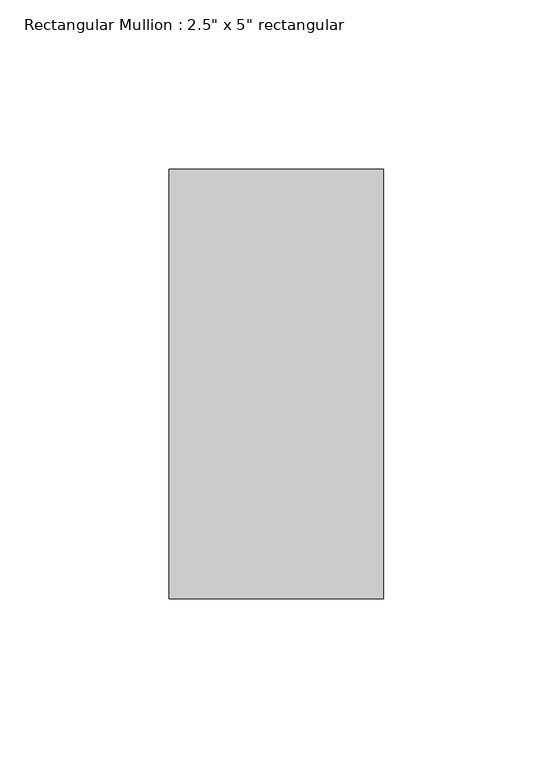
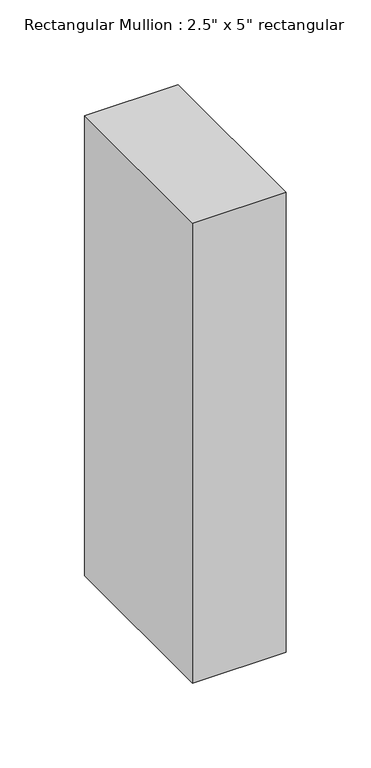
"""IFC4 building model written with IfcOpenShell, lengths in millimetres: member geometry."""

from ifc_helpers import new_model, si_unit, frame, origin, place, context, project, spatial, polyline, outline, extrude, source, transform, mapped, element, save


def member_ff9f2d30(model_context):
    return source(origin(), model_context, "Body", "SweptSolid", [
        extrude(outline(polyline([(0.0, 63.5), (0.0, -63.5), (-63.5, -63.5), (-63.5, 63.5), (0.0, 63.5)])), frame((0.0, 0.0, -330.2), z_axis=(0.0, 0.0, 1.0), x_axis=(1.0, 0.0, 0.0)), (0.0, 0.0, 1.0), 330.2),
    ])


if __name__ == "__main__":
    model = new_model("IFC4")
    model_context = context("Model", 3, world=origin())
    ifc_project = project(units=[si_unit("LENGTHUNIT", "METRE", prefix="MILLI")], contexts=[model_context])
    site = spatial("IfcSite", under=ifc_project)
    building = spatial("IfcBuilding", under=site)
    placement = place(None, origin())
    member_shape = member_ff9f2d30(model_context)
    element("IfcMember", 1, ObjectType="Rectangular Mullion : 2.5\" x 5\" rectangular", at=placement, inside=building, context=model_context, shape_type="MappedRepresentation", body=[
        mapped(member_shape, transform((0.0, 0.0, 0.0), x_axis=(1.0, 0.0, 0.0), y_axis=(0.0, 1.0, 0.0), z_axis=(0.0, 0.0, 1.0))),
    ])
    save(model, "model.ifc")

# Revit data of these elements
# Type "Rectangular Mullion : 2.5\" x 5\" rectangular"
#   built-in parameter 1007304 = 0.416667 (stored number, unit not read)
#   built-in parameter 1007301 = 0.104167 (stored number, unit not read)
#   built-in parameter 1007300 = 0.104167 (stored number, unit not read)
